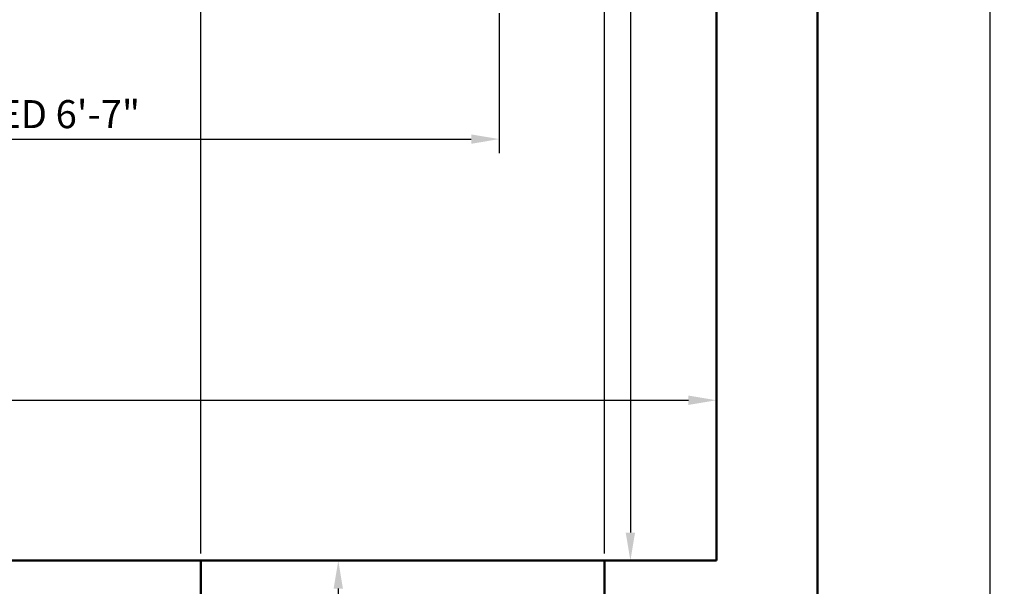
# Model space of a CAD drawing. Units: inches. Extents: x 2385 to 2740, y 1752 to 2305.
# Tile 5 of 15: x 2641 to 2729, y 1861 to 1911. Entities that reach past the tile are written whole.
import ezdxf

# ---------------------------------------------------------------- set-up
doc = ezdxf.new("R2010")
doc.units = ezdxf.units.IN
doc.layers.add('A-ANNO-DIMS', color=2, linetype='Continuous', lineweight=18)
doc.layers.add('A-WALL', color=7, linetype='Continuous', lineweight=50)
doc.styles.get("Standard").update_dxf_attribs({"font": 'arial.ttf'})
doc.dimstyles.new('Copy of ISO-25', dxfattribs={"dimtxt": 2.5, "dimasz": 2.5, "dimexe": 1.25, "dimexo": 0.625, "dimtad": 1, "dimdec": 1, "dimlunit": 4, "dimtxsty": 'Standard', "dimcen": 2.5, "dimadec": 0, "dimazin": 0, "dimtfac": 1, "dimtdec": 1, "dimtmove": 0, "dimatfit": 3, "dimfxl": 1, "dimarcsym": 0})

# ---------------------------------------------------------------- blocks, each defined once
blk = doc.blocks.new('*D16')
at = {"layer": 'A-ANNO-DIMS', "color": 0, "lineweight": -2, "transparency": 16777216}
for p, q in [((2559.248, 1863.595), (2559.248, 1878.516)), ((2703.248, 1863.595), (2703.248, 1878.516)), ((2561.748, 1877.266), (2700.748, 1877.266))]:
    blk.add_line(p, q, dxfattribs=at)
at = {"layer": 'A-ANNO-DIMS', "color": 0, "transparency": 16777216}
for points in [[(2561.748, 1877.683), (2561.748, 1876.849), (2559.248, 1877.266)], [(2700.748, 1877.683), (2700.748, 1876.849), (2703.248, 1877.266)]]:
    blk.add_solid(points, dxfattribs=at)
at = {"layer": 'Defpoints', "color": 0, "transparency": 16777216}
for p in [(2703.248, 1877.266), (2559.248, 1862.97), (2703.248, 1862.97)]:
    blk.add_point(p, dxfattribs=at)
at = {"layer": 'A-ANNO-DIMS', "color": 0, "transparency": 16777216, "insert": (2631.248, 1879.146), "char_height": 2.5, "attachment_point": 5}
blk.add_mtext("12'", dxfattribs=at)
blk = doc.blocks.new('*D17')
at = {"layer": 'A-ANNO-DIMS', "color": 0, "lineweight": -2, "transparency": 16777216}
for p, q in [((2702.623, 1978.97), (2694.318, 1978.97)), ((2695.568, 1976.47), (2695.568, 1865.47)), ((2702.623, 1862.97), (2694.318, 1862.97))]:
    blk.add_line(p, q, dxfattribs=at)
at = {"layer": 'A-ANNO-DIMS', "color": 0, "transparency": 16777216}
for points in [[(2695.152, 1976.47), (2695.985, 1976.47), (2695.568, 1978.97)], [(2695.152, 1865.47), (2695.985, 1865.47), (2695.568, 1862.97)]]:
    blk.add_solid(points, dxfattribs=at)
at = {"layer": 'Defpoints', "color": 0, "transparency": 16777216}
for p in [(2703.248, 1978.97), (2695.568, 1862.97), (2703.248, 1862.97)]:
    blk.add_point(p, dxfattribs=at)
at = {"layer": 'A-ANNO-DIMS', "color": 0, "transparency": 16777216, "insert": (2693.667, 1920.97), "char_height": 2.5, "attachment_point": 5, "rotation": 90}
blk.add_mtext('9\'-8"', dxfattribs=at)
blk = doc.blocks.new('*D18')
at = {"layer": 'A-ANNO-DIMS', "color": 0, "lineweight": -2, "transparency": 16777216}
for p, q in [((2657.873, 1862.97), (2670.757, 1862.97)), ((2669.507, 1860.47), (2669.507, 1787.47)), ((2657.873, 1784.97), (2670.757, 1784.97))]:
    blk.add_line(p, q, dxfattribs=at)
at = {"layer": 'A-ANNO-DIMS', "color": 0, "transparency": 16777216}
for points in [[(2669.091, 1860.47), (2669.924, 1860.47), (2669.507, 1862.97)], [(2669.091, 1787.47), (2669.924, 1787.47), (2669.507, 1784.97)]]:
    blk.add_solid(points, dxfattribs=at)
at = {"layer": 'Defpoints', "color": 0, "transparency": 16777216}
for p in [(2657.248, 1862.97), (2657.248, 1784.97), (2669.507, 1784.97)]:
    blk.add_point(p, dxfattribs=at)
at = {"layer": 'A-ANNO-DIMS', "color": 0, "transparency": 16777216, "insert": (2667.606, 1823.97), "char_height": 2.5, "attachment_point": 5, "rotation": 90}
blk.add_mtext('6\'-6"', dxfattribs=at)
blk = doc.blocks.new('*D25')
at = {"layer": 'A-ANNO-DIMS', "color": 0, "lineweight": -2, "transparency": 16777216}
for p, q in [((2712.873, 2275.97), (2728.926, 2275.97)), ((2727.676, 1781.47), (2727.676, 2273.47)), ((2712.873, 1778.97), (2728.926, 1778.97))]:
    blk.add_line(p, q, dxfattribs=at)
at = {"layer": 'A-ANNO-DIMS', "color": 0, "transparency": 16777216}
for points in [[(2727.259, 2273.47), (2728.092, 2273.47), (2727.676, 2275.97)], [(2727.259, 1781.47), (2728.092, 1781.47), (2727.676, 1778.97)]]:
    blk.add_solid(points, dxfattribs=at)
at = {"layer": 'Defpoints', "color": 0, "transparency": 16777216}
for p in [(2712.248, 2275.97), (2727.676, 2275.97), (2712.248, 1778.97)]:
    blk.add_point(p, dxfattribs=at)
at = {"layer": 'A-ANNO-DIMS', "color": 0, "transparency": 16777216, "insert": (2725.774, 2027.47), "char_height": 2.5, "attachment_point": 5, "rotation": 90}
blk.add_mtext('41\'-5"', dxfattribs=at)
blk = doc.blocks.new('*D28')
at = {"layer": 'A-ANNO-DIMS', "color": 0, "lineweight": -2, "transparency": 16777216}
for p, q in [((2604.89, 1911.766), (2604.89, 1899.294)), ((2683.867, 1911.766), (2683.867, 1899.294)), ((2607.39, 1900.544), (2681.367, 1900.544))]:
    blk.add_line(p, q, dxfattribs=at)
at = {"layer": 'A-ANNO-DIMS', "color": 0, "transparency": 16777216}
for points in [[(2607.39, 1900.961), (2607.39, 1900.127), (2604.89, 1900.544)], [(2681.367, 1900.961), (2681.367, 1900.127), (2683.867, 1900.544)]]:
    blk.add_solid(points, dxfattribs=at)
at = {"layer": 'Defpoints', "color": 0, "transparency": 16777216}
for p in [(2604.89, 1912.391), (2683.867, 1912.391), (2683.867, 1900.544)]:
    blk.add_point(p, dxfattribs=at)
at = {"layer": 'A-ANNO-DIMS', "color": 0, "transparency": 16777216, "insert": (2644.378, 1902.445), "char_height": 2.5, "attachment_point": 5}
blk.add_mtext('BED 6\'-7"', dxfattribs=at)
blk = doc.blocks.new('*D43')
at = {"layer": 'A-ANNO-DIMS', "color": 0, "lineweight": -2, "transparency": 16777216}
for p, q in [((2657.248, 1863.595), (2657.248, 2302.837)), ((2693.248, 1863.595), (2693.248, 2302.837)), ((2659.748, 2301.587), (2690.748, 2301.587))]:
    blk.add_line(p, q, dxfattribs=at)
at = {"layer": 'A-ANNO-DIMS', "color": 0, "transparency": 16777216}
for points in [[(2659.748, 2302.004), (2659.748, 2301.171), (2657.248, 2301.587)], [(2690.748, 2302.004), (2690.748, 2301.171), (2693.248, 2301.587)]]:
    blk.add_solid(points, dxfattribs=at)
at = {"layer": 'Defpoints', "color": 0, "transparency": 16777216}
for p in [(2693.248, 2301.587), (2657.248, 1862.97), (2693.248, 1862.97)]:
    blk.add_point(p, dxfattribs=at)
at = {"layer": 'A-ANNO-DIMS', "color": 0, "transparency": 16777216, "insert": (2675.248, 2303.49), "char_height": 2.5, "attachment_point": 5}
blk.add_mtext('3\'-0"', dxfattribs=at)

msp = doc.modelspace()

# ---------------------------------------------------------------- linework, layer by layer
at = {"layer": 'A-WALL'}
for p, q in [((2712.248, 2275.97), (2712.248, 1778.97)), ((2703.248, 1978.97), (2703.248, 1862.97)), ((2703.248, 1978.97), (2703.248, 1862.97)), ((2712.248, 1978.97), (2712.248, 1862.97)), ((2657.248, 1862.97), (2559.248, 1862.97)), ((2657.248, 1856.97), (2657.248, 1862.97)), ((2657.248, 1862.97), (2693.248, 1862.97)), ((2703.248, 1862.97), (2693.248, 1862.97)), ((2693.248, 1856.97), (2693.248, 1862.97)), ((2712.248, 1862.97), (2712.248, 1778.97))]:
    msp.add_line(p, q, dxfattribs=at)

# ---------------------------------------------------------------- dimensions: what is measured, and where the dimension line sits
at = {"layer": 'A-ANNO-DIMS'}
for base, p1, p2, override, picture, middle in [((2693.248, 2301.587), (2657.248, 1862.97), (2693.248, 1862.97), {"dimdec": 1, "dimlfac": 1, "dimrnd": 0, "dimzin": 1, "dimdsep": 46, "dimlunit": 4, "dimfrac": 2}, '*D43', (2675.248, 2303.49)), ((2703.248, 1877.266), (2559.248, 1862.97), (2703.248, 1862.97), {"dimclrd": 0, "dimclre": 0, "dimclrt": 0}, '*D16', (2631.248, 1879.146))]:
    dim = msp.add_linear_dim(base=base, p1=p1, p2=p2, dimstyle='Copy of ISO-25', override=override, dxfattribs=at)
    dim.commit()
    dim.dimension.update_dxf_attribs({"geometry": picture, "text_midpoint": middle})
for base, p1, p2, picture, middle in [((2727.676, 2275.97), (2712.248, 1778.97), (2712.248, 2275.97), '*D25', (2725.774, 2027.47)), ((2695.568, 1862.97), (2703.248, 1978.97), (2703.248, 1862.97), '*D17', (2693.667, 1920.97)), ((2669.507, 1784.97), (2657.248, 1862.97), (2657.248, 1784.97), '*D18', (2667.606, 1823.97))]:
    dim = msp.add_linear_dim(base=base, p1=p1, p2=p2, angle=90, dimstyle='Copy of ISO-25', override={"dimclrd": 0, "dimclre": 0, "dimclrt": 0}, dxfattribs=at)
    dim.commit()
    dim.dimension.update_dxf_attribs({"geometry": picture, "text_midpoint": middle})
dim = msp.add_linear_dim(base=(2683.867, 1900.544), p1=(2604.89, 1912.391), p2=(2683.867, 1912.391), text='BED <>', dimstyle='Copy of ISO-25', override={"dimdec": 1, "dimlfac": 1, "dimrnd": 0, "dimzin": 1, "dimdsep": 46, "dimlunit": 4, "dimfrac": 2}, dxfattribs=at)
dim.commit()
dim.dimension.update_dxf_attribs({"geometry": '*D28', "text_midpoint": (2644.378, 1902.445)})

doc.saveas('drawing.dxf')
